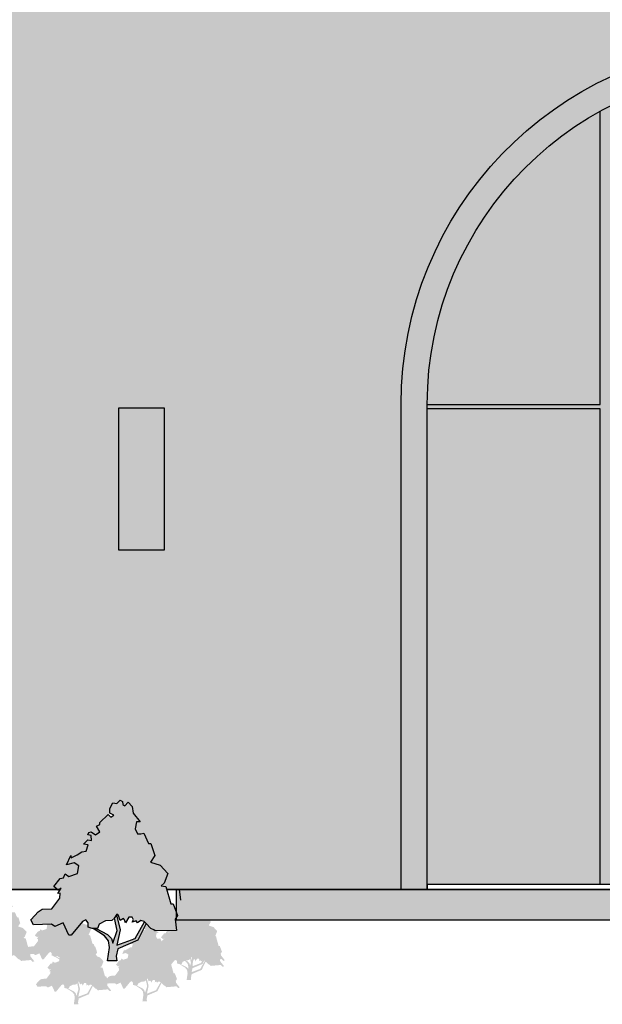
# Model space of a CAD drawing. Units: feet. Extents: x 2368 to 3224, y 836 to 1229.
# Tile 6 of 9: x 2515 to 2603, y 836 to 985. Entities that reach past the tile are written whole.
import ezdxf

# ---------------------------------------------------------------- set-up
doc = ezdxf.new("R2010")
doc.units = ezdxf.units.FT
for name, color, linetype, lineweight in [('A-ELEV', 7, 'Continuous', 25), ('A-ELEV-PATT', 8, 'Continuous', 13), ('L-PLNT', 3, 'Continuous', 13)]:
    doc.layers.add(name, color=color, linetype=linetype, lineweight=lineweight)

msp = doc.modelspace()

# ---------------------------------------------------------------- hatches: boundary and pattern name
at = {"layer": 'A-ELEV-PATT'}
h = msp.add_hatch(color=256, dxfattribs=at)
h.dxf.hatch_style = 1
h.paths.add_polyline_path([(2584.6, 1202.15), (2582.11, 1202.15), (2582.11, 1108.75), (2584.6, 1108.75)])
h.paths.add_polyline_path([(2656.21, 1202.15), (2653.72, 1202.15), (2653.72, 1108.75), (2656.21, 1108.75)])
h.paths.add_polyline_path([(2693.73, 1040.78), (2656.21, 1040.78), (2656.21, 1099.51), (2653.72, 1099.51), (2653.72, 1040.78), (2584.6, 1040.78), (2584.6, 1099.51), (2582.11, 1099.51), (2582.11, 1040.78), (2544.98, 1040.78), (2544.98, 1040.06), (2582.11, 1040.06), (2582.11, 1037.14), (2544.98, 1037.14), (2544.98, 1036.77), (2582.11, 1036.77), (2582.11, 1033.48), (2544.98, 1033.48), (2544.98, 1033.11), (2582.11, 1033.11), (2582.11, 1029.83), (2544.98, 1029.83), (2544.98, 1029.46), (2582.11, 1029.46), (2582.11, 1026.18), (2544.98, 1026.18), (2544.98, 1025.81), (2582.11, 1025.81), (2582.11, 1022.52), (2544.98, 1022.52), (2544.98, 1022.15), (2582.11, 1022.15), (2582.11, 1018.87), (2544.98, 1018.87), (2544.98, 1018.5), (2582.11, 1018.5), (2582.11, 1015.21), (2544.98, 1015.21), (2544.98, 1014.84), (2582.11, 1014.84), (2582.11, 1011.56), (2544.98, 1011.56), (2544.98, 1011.19), (2582.11, 1011.19), (2582.11, 1007.9), (2544.98, 1007.9), (2544.98, 1007.53), (2582.11, 1007.53), (2582.11, 1006.11), (2584.6, 1006.11), (2584.6, 1007.53), (2619.49, 1007.53), (2619.49, 1006.11), (2620.43, 1006.11), (2620.43, 1007.53), (2653.72, 1007.53), (2653.72, 1006.11), (2656.21, 1006.11), (2656.21, 1007.53), (2693.73, 1007.53), (2693.73, 1007.9), (2656.21, 1007.9), (2656.21, 1011.19), (2693.73, 1011.19), (2693.73, 1011.56), (2656.21, 1011.56), (2656.21, 1014.84), (2693.73, 1014.84), (2693.73, 1015.21), (2656.21, 1015.21), (2656.21, 1018.5), (2693.73, 1018.5), (2693.73, 1018.87), (2656.21, 1018.87), (2656.21, 1022.15), (2693.73, 1022.15), (2693.73, 1022.52), (2656.21, 1022.52), (2656.21, 1025.81), (2693.73, 1025.81), (2693.73, 1026.18), (2656.21, 1026.18), (2656.21, 1029.46), (2693.73, 1029.46), (2693.73, 1029.83), (2656.21, 1029.83), (2656.21, 1033.11), (2693.73, 1033.11), (2693.73, 1033.48), (2656.21, 1033.48), (2656.21, 1036.77), (2693.73, 1036.77), (2693.73, 1037.14), (2656.21, 1037.14), (2656.21, 1040.06), (2693.73, 1040.06)])
h.paths.add_polyline_path([(2584.6, 1040.06), (2619.49, 1040.06), (2619.49, 1037.14), (2584.6, 1037.14)], flags=16)
h.paths.add_polyline_path([(2584.6, 1036.77), (2619.49, 1036.77), (2619.49, 1033.48), (2584.6, 1033.48)], flags=16)
h.paths.add_polyline_path([(2584.6, 1033.11), (2619.49, 1033.11), (2619.49, 1029.83), (2584.6, 1029.83)], flags=16)
h.paths.add_polyline_path([(2584.6, 1029.46), (2619.49, 1029.46), (2619.49, 1026.18), (2584.6, 1026.18)], flags=16)
h.paths.add_polyline_path([(2584.6, 1025.81), (2619.49, 1025.81), (2619.49, 1022.52), (2584.6, 1022.52)], flags=16)
h.paths.add_polyline_path([(2584.6, 1022.15), (2619.49, 1022.15), (2619.49, 1018.87), (2584.6, 1018.87)], flags=16)
h.paths.add_polyline_path([(2584.6, 1018.5), (2619.49, 1018.5), (2619.49, 1015.21), (2584.6, 1015.21)], flags=16)
h.paths.add_polyline_path([(2584.6, 1014.84), (2619.49, 1014.84), (2619.49, 1011.56), (2584.6, 1011.56)], flags=16)
h.paths.add_polyline_path([(2584.6, 1011.19), (2619.49, 1011.19), (2619.49, 1007.9), (2584.6, 1007.9)], flags=16)
h.paths.add_polyline_path([(2620.43, 1040.06), (2653.72, 1040.06), (2653.72, 1037.14), (2620.43, 1037.14)], flags=16)
h.paths.add_polyline_path([(2620.43, 1036.77), (2653.72, 1036.77), (2653.72, 1033.48), (2620.43, 1033.48)], flags=16)
h.paths.add_polyline_path([(2620.43, 1033.11), (2653.72, 1033.11), (2653.72, 1029.83), (2620.43, 1029.83)], flags=16)
h.paths.add_polyline_path([(2620.43, 1029.46), (2653.72, 1029.46), (2653.72, 1026.18), (2620.43, 1026.18)], flags=16)
h.paths.add_polyline_path([(2620.43, 1025.81), (2653.72, 1025.81), (2653.72, 1022.52), (2620.43, 1022.52)], flags=16)
h.paths.add_polyline_path([(2620.43, 1022.15), (2653.72, 1022.15), (2653.72, 1018.87), (2620.43, 1018.87)], flags=16)
h.paths.add_polyline_path([(2620.43, 1018.5), (2653.72, 1018.5), (2653.72, 1015.21), (2620.43, 1015.21)], flags=16)
h.paths.add_polyline_path([(2620.43, 1014.84), (2653.72, 1014.84), (2653.72, 1011.56), (2620.43, 1011.56)], flags=16)
h.paths.add_polyline_path([(2620.43, 1011.19), (2653.72, 1011.19), (2653.72, 1007.9), (2620.43, 1007.9)], flags=16)
h.paths.add_polyline_path([(2536.7, 926.19), (2529.87, 926.19), (2529.87, 904.71), (2536.7, 904.71)])
h.paths.add_polyline_path([(2422.21, 920.11), (2416.4, 920.11), (2416.4, 905.78), (2422.21, 905.78)])
h = msp.add_hatch(color=256, dxfattribs=at)
h.dxf.hatch_style = 1
h.paths.add_polyline_path([(2452.58, 1176.09), (2421.63, 1176.09), (2421.63, 1113.35), (2452.58, 1113.35)])
h.paths.add_polyline_path([(2483.52, 1113.35), (2452.58, 1113.35), (2452.58, 1050.6), (2483.52, 1050.6)])
h.paths.add_polyline_path([(2452.58, 1050.6), (2421.63, 1050.6), (2421.63, 987.86), (2452.58, 987.86)])
h.paths.add_polyline_path([(2536.7, 926.19), (2536.7, 904.71), (2529.87, 904.71), (2529.87, 926.19)], flags=16)
h.paths.add_polyline_path([(2719.16, 1202.15), (2694.93, 1202.15), (2694.93, 1108.75), (2694.93, 1002.87), (2696.85, 1002.87), (2696.85, 987.86), (2719.16, 987.86)])
h = msp.add_hatch(color=256, dxfattribs=at)
h.dxf.hatch_style = 1
h.paths.add_polyline_path([(2582.11, 1191.22), (2544.98, 1191.22), (2544.98, 1108.75), (2582.11, 1108.75)])
h.paths.add_polyline_path([(2653.72, 1191.22), (2584.6, 1191.22), (2584.6, 1108.75), (2653.72, 1108.75)])
h.paths.add_polyline_path([(2693.73, 1191.22), (2656.21, 1191.22), (2656.21, 1108.75), (2693.73, 1108.75)])
h.paths.add_polyline_path([(2653.72, 1099.51), (2584.6, 1099.51), (2584.6, 1040.78), (2653.72, 1040.78)])
h.paths.add_polyline_path([(2693.73, 1099.51), (2656.21, 1099.51), (2656.21, 1040.78), (2693.73, 1040.78)])
h.paths.add_polyline_path([(2582.11, 1099.51), (2544.98, 1099.51), (2544.98, 1040.78), (2582.11, 1040.78)])
h.paths.add_polyline_path([(2582.11, 1036.77), (2544.98, 1036.77), (2544.98, 1033.48), (2582.11, 1033.48)])
h.paths.add_polyline_path([(2582.11, 1033.11), (2544.98, 1033.11), (2544.98, 1029.83), (2582.11, 1029.83)])
h.paths.add_polyline_path([(2582.11, 1029.46), (2544.98, 1029.46), (2544.98, 1026.18), (2582.11, 1026.18)])
h.paths.add_polyline_path([(2582.11, 1025.81), (2544.98, 1025.81), (2544.98, 1022.52), (2582.11, 1022.52)])
h.paths.add_polyline_path([(2582.11, 1022.15), (2544.98, 1022.15), (2544.98, 1018.87), (2582.11, 1018.87)])
h.paths.add_polyline_path([(2582.11, 1018.5), (2544.98, 1018.5), (2544.98, 1015.21), (2582.11, 1015.21)])
h.paths.add_polyline_path([(2582.11, 1007.53), (2544.98, 1007.53), (2544.98, 1006.11), (2582.11, 1006.11)])
h.paths.add_polyline_path([(2582.11, 1011.19), (2544.98, 1011.19), (2544.98, 1007.9), (2582.11, 1007.9)])
h.paths.add_polyline_path([(2582.11, 1014.84), (2544.98, 1014.84), (2544.98, 1011.56), (2582.11, 1011.56)])
h.paths.add_polyline_path([(2619.49, 1007.53), (2584.6, 1007.53), (2584.6, 1006.11), (2619.49, 1006.11)])
h.paths.add_polyline_path([(2619.49, 1011.19), (2584.6, 1011.19), (2584.6, 1007.9), (2619.49, 1007.9)])
h.paths.add_polyline_path([(2619.49, 1014.84), (2584.6, 1014.84), (2584.6, 1011.56), (2619.49, 1011.56)])
h.paths.add_polyline_path([(2619.49, 1018.5), (2584.6, 1018.5), (2584.6, 1015.21), (2619.49, 1015.21)])
h.paths.add_polyline_path([(2619.49, 1022.15), (2584.6, 1022.15), (2584.6, 1018.87), (2619.49, 1018.87)])
h.paths.add_polyline_path([(2619.49, 1025.81), (2584.6, 1025.81), (2584.6, 1022.52), (2619.49, 1022.52)])
h.paths.add_polyline_path([(2619.49, 1029.46), (2584.6, 1029.46), (2584.6, 1026.18), (2619.49, 1026.18)])
h.paths.add_polyline_path([(2619.49, 1033.11), (2584.6, 1033.11), (2584.6, 1029.83), (2619.49, 1029.83)])
h.paths.add_polyline_path([(2619.49, 1036.77), (2584.6, 1036.77), (2584.6, 1033.48), (2619.49, 1033.48)])
h.paths.add_polyline_path([(2582.11, 1040.06), (2544.98, 1040.06), (2544.98, 1037.14), (2582.11, 1037.14)])
h.paths.add_polyline_path([(2619.49, 1040.06), (2584.6, 1040.06), (2584.6, 1037.14), (2619.49, 1037.14)])
h.paths.add_polyline_path([(2653.72, 1040.06), (2620.43, 1040.06), (2620.43, 1037.14), (2653.72, 1037.14)])
h.paths.add_polyline_path([(2653.72, 1036.77), (2620.43, 1036.77), (2620.43, 1033.48), (2653.72, 1033.48)])
h.paths.add_polyline_path([(2653.72, 1033.11), (2620.43, 1033.11), (2620.43, 1029.83), (2653.72, 1029.83)])
h.paths.add_polyline_path([(2653.72, 1029.46), (2620.43, 1029.46), (2620.43, 1026.18), (2653.72, 1026.18)])
h.paths.add_polyline_path([(2653.72, 1025.81), (2620.43, 1025.81), (2620.43, 1022.52), (2653.72, 1022.52)])
h.paths.add_polyline_path([(2653.72, 1022.15), (2620.43, 1022.15), (2620.43, 1018.87), (2653.72, 1018.87)])
h.paths.add_polyline_path([(2653.72, 1018.5), (2620.43, 1018.5), (2620.43, 1015.21), (2653.72, 1015.21)])
h.paths.add_polyline_path([(2653.72, 1011.19), (2620.43, 1011.19), (2620.43, 1007.9), (2653.72, 1007.9)])
h.paths.add_polyline_path([(2653.72, 1014.84), (2620.43, 1014.84), (2620.43, 1011.56), (2653.72, 1011.56)])
h.paths.add_polyline_path([(2653.72, 1007.53), (2620.43, 1007.53), (2620.43, 1006.11), (2653.72, 1006.11)])
h.paths.add_polyline_path([(2693.73, 1007.53), (2656.21, 1007.53), (2656.21, 1006.11), (2693.73, 1006.11)])
h.paths.add_polyline_path([(2693.73, 1011.19), (2656.21, 1011.19), (2656.21, 1007.9), (2693.73, 1007.9)])
h.paths.add_polyline_path([(2693.73, 1014.84), (2656.21, 1014.84), (2656.21, 1011.56), (2693.73, 1011.56)])
h.paths.add_polyline_path([(2693.73, 1018.5), (2656.21, 1018.5), (2656.21, 1015.21), (2693.73, 1015.21)])
h.paths.add_polyline_path([(2693.73, 1022.15), (2656.21, 1022.15), (2656.21, 1018.87), (2693.73, 1018.87)])
h.paths.add_polyline_path([(2693.73, 1025.81), (2656.21, 1025.81), (2656.21, 1022.52), (2693.73, 1022.52)])
h.paths.add_polyline_path([(2693.73, 1029.46), (2656.21, 1029.46), (2656.21, 1026.18), (2693.73, 1026.18)])
h.paths.add_polyline_path([(2693.73, 1033.11), (2656.21, 1033.11), (2656.21, 1029.83), (2693.73, 1029.83)])
h.paths.add_polyline_path([(2693.73, 1040.06), (2656.21, 1040.06), (2656.21, 1037.14), (2693.73, 1037.14)])
h.paths.add_polyline_path([(2693.73, 1036.77), (2656.21, 1036.77), (2656.21, 1033.48), (2693.73, 1033.48)])
h.paths.add_polyline_path([(2510.02, 968.65), (2451.35, 968.65), (2451.35, 916.99), (2510.02, 916.99)])
h.paths.add_polyline_path([(2510.02, 916.99), (2470.8, 916.99), (2470.8, 861.76), (2510.02, 861.76)])
h.paths.add_polyline_path([(2650.82, 971.36, 0.250141), (2603.19, 971.36), (2603.19, 926.73), (2650.82, 926.73)])
h.paths.add_polyline_path([(2651.5, 971), (2651.5, 926.73), (2677.6, 926.73, 0.272847)])
h.paths.add_polyline_path([(2677.6, 926.06), (2651.5, 926.06), (2651.5, 854.24), (2677.6, 854.24)])
h.paths.add_polyline_path([(2650.82, 926.06), (2603.19, 926.06), (2603.19, 854.24), (2650.82, 854.24)])
h.paths.add_polyline_path([(2602.51, 971, 0.272847), (2576.42, 926.73), (2602.51, 926.73)])
h.paths.add_polyline_path([(2602.51, 926.06), (2576.42, 926.06), (2576.42, 854.24), (2602.51, 854.24)])
h = msp.add_hatch(color=256, dxfattribs=at)
h.dxf.hatch_style = 1
h.paths.add_polyline_path([(2624.92, 981.22), (2624.92, 981.73, -0.018787), (2629.09, 981.73), (2629.09, 981.22, -0.403049), (2681.53, 926.73), (2681.53, 853.51), (2701.14, 853.51), (2719.16, 853.51), (2719.16, 987.86), (2694.93, 987.86), (2544.98, 987.86), (2510.02, 987.86), (2510.02, 853.51), (2520.58, 853.51), (2520.05, 853.96), (2521, 855.17), (2521.51, 855.27), (2521.73, 855.83), (2522.31, 855.46), (2523.63, 855.92), (2523.84, 857.04), (2523.12, 857.51), (2521.95, 857.23), (2522.6, 858.63), (2522.68, 858.26), (2523.55, 858.73), (2524.28, 859.19), (2524.94, 859.29), (2525.23, 860.22), (2524.5, 860.32), (2525.17, 860.97), (2525.74, 860.88), (2525.67, 861.62), (2525.16, 861.72), (2525.3, 862.09), (2525.67, 862.19), (2526.32, 861.72), (2526.98, 862.19), (2526.47, 863.03), (2526.98, 863.31), (2526.98, 863.59), (2528.51, 865.09), (2528.51, 865.74), (2528.95, 866.58), (2529.53, 866.48), (2530.04, 866.95), (2530.41, 866.77), (2530.48, 866.3), (2530.77, 866.11), (2531.28, 866.67), (2531.86, 866.03), (2532.01, 864.99), (2533.1, 863.68), (2532.52, 863.68), (2532.3, 862.65), (2532.67, 861.9), (2533.18, 861.9), (2533.61, 862), (2534.34, 860.41), (2534.71, 860.41), (2535.29, 858.63), (2534.63, 857.61), (2536.09, 857.14), (2537.26, 855.92), (2536.52, 854.02), (2536.97, 853.96), (2537.09, 853.51), (2572.48, 853.51), (2572.48, 926.73, -0.403049)])
h.paths.add_polyline_path([(2536.7, 926.19), (2536.7, 904.71), (2529.87, 904.71), (2529.87, 926.19)], flags=16)
h = msp.add_hatch(color=256, dxfattribs=at)
h.dxf.hatch_style = 1
h.paths.add_polyline_path([(2624.92, 981.22, 0.403049), (2572.48, 926.73), (2572.48, 853.51), (2576.42, 853.51), (2576.42, 926.73, -0.402184), (2624.92, 977.28)])
h.paths.add_polyline_path([(2629.09, 981.22), (2629.09, 977.28, -0.402184), (2677.6, 926.73), (2677.6, 853.51), (2681.53, 853.51), (2681.53, 926.73, 0.403049)])
h.paths.add_polyline_path([(2629.09, 981.22), (2629.09, 981.73, 0.018787), (2624.92, 981.73), (2624.92, 977.28, -0.020626), (2629.09, 977.28)])
h = msp.add_hatch(color=256, dxfattribs=at)
h.dxf.hatch_style = 1
h.paths.add_polyline_path([(2603.19, 971.36, 0.00378), (2602.51, 971), (2602.51, 926.73), (2576.42, 926.73), (2576.42, 926.06), (2602.51, 926.06), (2602.51, 854.24), (2603.19, 854.24), (2603.19, 926.06), (2650.82, 926.06), (2650.82, 854.24), (2651.5, 854.24), (2651.5, 926.06), (2677.6, 926.06), (2677.6, 926.73), (2651.5, 926.73), (2651.5, 971, 0.00378), (2650.82, 971.36), (2650.82, 926.73), (2603.19, 926.73)])
h = msp.add_hatch(color=256, dxfattribs=at)
h.dxf.hatch_style = 1
h.paths.add_polyline_path([(2536.7, 926.19), (2536.7, 904.71), (2529.87, 904.71), (2529.87, 926.19)], flags=16)
h = msp.add_hatch(color=256, dxfattribs=at)
h.dxf.hatch_style = 1
h.paths.add_polyline_path([(2701.14, 853.51), (2538.51, 853.51), (2538.51, 848.93), (2701.14, 848.93)])
at = {"layer": 'L-PLNT'}
h = msp.add_hatch(color=256, dxfattribs=at)
h.dxf.hatch_style = 1
h.paths.add_polyline_path([(2536.97, 853.96), (2536.24, 854.05), (2536.68, 854.43), (2537.26, 855.92), (2536.09, 857.14), (2534.63, 857.61), (2535.29, 858.63), (2534.71, 860.41), (2534.34, 860.41), (2533.61, 862), (2533.18, 861.9), (2532.67, 861.9), (2532.3, 862.65), (2532.52, 863.68), (2533.1, 863.68), (2532.01, 864.99), (2531.86, 866.03), (2531.28, 866.67), (2530.77, 866.11), (2530.48, 866.3), (2530.41, 866.77), (2530.04, 866.95), (2529.53, 866.48), (2528.95, 866.58), (2528.51, 865.74), (2528.51, 864.99), (2529.09, 864.71), (2528.66, 864.43), (2528.22, 864.8), (2526.98, 863.59), (2526.98, 863.31), (2526.47, 863.03), (2526.98, 862.19), (2526.32, 861.72), (2525.67, 862.19), (2525.3, 862.09), (2525.16, 861.72), (2525.67, 861.62), (2525.74, 860.88), (2525.17, 860.97), (2524.5, 860.32), (2525.23, 860.22), (2524.94, 859.29), (2524.28, 859.19), (2523.55, 858.73), (2522.68, 858.26), (2522.6, 858.63), (2521.95, 857.23), (2523.12, 857.51), (2523.84, 857.04), (2523.63, 855.92), (2522.31, 855.46), (2521.73, 855.83), (2521.51, 855.27), (2521, 855.17), (2520.05, 853.96), (2520.58, 853.51), (2520.88, 853.51), (2521.15, 853.68), (2520.65, 852.87), (2521.01, 852.91), (2520.96, 852.17), (2519.76, 850.59), (2518.3, 850.5), (2517.65, 850.13), (2516.55, 848.91), (2516.99, 848.16), (2519.69, 848.26), (2520.2, 847.88), (2521.44, 848.44), (2522.31, 846.58), (2522.68, 846.58), (2524.35, 848.63), (2524.87, 848.91), (2525.23, 848.44), (2525.23, 847.79), (2525.81, 847.6), (2526.61, 847.6), (2526.91, 848.26), (2527.85, 848.73), (2528.8, 848.82), (2529.22, 849.18), (2529.31, 849.29), (2529.53, 849.75), (2529.82, 849.57), (2530.04, 848.82), (2530.55, 849.1), (2530.7, 848.91), (2530.84, 848.44), (2531.35, 849.29), (2531.86, 849.29), (2532.23, 848.66), (2532.45, 848.73), (2532.67, 848.44), (2533.18, 848.82), (2533.73, 848.61), (2533.72, 848.6), (2533.98, 848.35), (2534.71, 847.6), (2535.15, 847.42), (2535.33, 847.23), (2538.57, 847.32), (2538.35, 849.01), (2538.51, 849.24), (2538.51, 850.13), (2538.06, 851.34), (2537.7, 851.34)])
h = msp.add_hatch(color=256, dxfattribs=at)
h.dxf.hatch_style = 1
h.paths.add_polyline_path([(2515.94, 847.08), (2515.36, 847.68), (2514.64, 847.91), (2514.97, 848.41), (2514.68, 849.29), (2514.5, 849.29), (2514.14, 850.07), (2513.93, 850.03), (2513.67, 850.03), (2513.49, 850.4), (2513.6, 850.9), (2513.89, 850.9), (2513.35, 851.55), (2513.28, 852.06), (2512.99, 852.38), (2512.74, 852.1), (2512.6, 852.19), (2512.56, 852.42), (2512.38, 852.52), (2512.13, 852.29), (2511.84, 852.33), (2511.62, 851.92), (2511.62, 851.55), (2511.91, 851.41), (2511.7, 851.27), (2511.48, 851.46), (2510.87, 850.86), (2510.87, 850.72), (2510.62, 850.58), (2510.69, 850.44), (2510.87, 850.17), (2510.55, 849.94), (2510.22, 850.17), (2510.04, 850.12), (2509.97, 849.94), (2510.22, 849.89), (2510.26, 849.52), (2509.98, 849.57), (2509.65, 849.24), (2510.01, 849.2), (2509.86, 848.74), (2509.54, 848.69), (2509.18, 848.46), (2508.75, 848.23), (2508.71, 848.41), (2508.39, 847.72), (2508.96, 847.86), (2509.32, 847.63), (2509.22, 847.08), (2508.57, 846.85), (2508.28, 847.03), (2508.17, 846.76), (2507.92, 846.71), (2507.71, 846.43), (2507.46, 846.11), (2507.78, 845.83), (2507.99, 845.97), (2507.75, 845.57), (2507.93, 845.59), (2507.9, 845.23), (2507.31, 844.45), (2506.59, 844.41), (2506.27, 844.22), (2505.73, 843.62), (2505.95, 843.25), (2507.28, 843.3), (2507.53, 843.12), (2508.14, 843.39), (2508.57, 842.47), (2508.75, 842.47), (2509.58, 843.48), (2509.83, 843.62), (2510.01, 843.39), (2510.01, 843.07), (2510.29, 842.98), (2510.69, 842.98), (2510.83, 843.3), (2511.3, 843.53), (2511.77, 843.58), (2511.98, 843.76), (2512.02, 843.81), (2512.13, 844.04), (2512.27, 843.94), (2512.38, 843.58), (2512.63, 843.71), (2512.7, 843.62), (2512.78, 843.39), (2513.03, 843.81), (2513.28, 843.81), (2513.39, 843.62), (2513.28, 843.44), (2513.57, 843.53), (2513.67, 843.39), (2513.93, 843.58), (2514.18, 843.48), (2514.68, 842.98), (2514.9, 842.88), (2515.08, 842.7), (2516.59, 842.84), (2516.87, 842.56), (2517.09, 842.65), (2516.51, 843.39), (2516.48, 843.67), (2516.66, 843.94), (2516.33, 844.82), (2516.15, 844.82), (2515.79, 846.11), (2515.43, 846.16), (2515.65, 846.34)])
h = msp.add_hatch(color=256, dxfattribs=at)
h.dxf.hatch_style = 1
h.paths.add_polyline_path([(2525.66, 847.53), (2525.09, 848.13), (2524.37, 848.36), (2524.69, 848.86), (2524.4, 849.74), (2524.22, 849.74), (2523.86, 850.52), (2523.65, 850.48), (2523.4, 850.48), (2523.22, 850.85), (2523.33, 851.35), (2523.61, 851.35), (2523.07, 852), (2523, 852.51), (2522.71, 852.83), (2522.46, 852.55), (2522.32, 852.64), (2522.28, 852.87), (2522.1, 852.97), (2521.85, 852.74), (2521.56, 852.78), (2521.35, 852.37), (2521.35, 852), (2521.64, 851.86), (2521.42, 851.72), (2521.2, 851.91), (2520.59, 851.31), (2520.59, 851.17), (2520.34, 851.03), (2520.41, 850.89), (2520.59, 850.62), (2520.27, 850.39), (2519.95, 850.62), (2519.77, 850.57), (2519.69, 850.39), (2519.95, 850.34), (2519.98, 849.97), (2519.7, 850.02), (2519.37, 849.69), (2519.73, 849.65), (2519.59, 849.19), (2519.26, 849.14), (2518.9, 848.91), (2518.47, 848.68), (2518.44, 848.86), (2518.11, 848.17), (2518.69, 848.31), (2519.05, 848.08), (2518.94, 847.53), (2518.29, 847.3), (2518.01, 847.48), (2517.9, 847.21), (2517.65, 847.16), (2517.43, 846.88), (2517.18, 846.56), (2517.5, 846.28), (2517.72, 846.42), (2517.47, 846.02), (2517.65, 846.04), (2517.63, 845.68), (2517.03, 844.9), (2516.32, 844.86), (2515.99, 844.67), (2515.45, 844.07), (2515.67, 843.7), (2517, 843.75), (2517.25, 843.57), (2517.86, 843.84), (2518.29, 842.92), (2518.47, 842.92), (2519.3, 843.93), (2519.55, 844.07), (2519.73, 843.84), (2519.73, 843.52), (2520.02, 843.43), (2520.41, 843.43), (2520.56, 843.75), (2521.02, 843.98), (2521.49, 844.03), (2521.71, 844.21), (2521.74, 844.26), (2521.85, 844.49), (2522, 844.39), (2522.1, 844.03), (2522.35, 844.16), (2522.43, 844.07), (2522.5, 843.84), (2522.75, 844.26), (2523, 844.26), (2523.11, 844.07), (2523, 843.89), (2523.29, 843.98), (2523.4, 843.84), (2523.65, 844.03), (2523.9, 843.93), (2524.4, 843.43), (2524.62, 843.33), (2524.8, 843.15), (2526.31, 843.29), (2526.6, 843.01), (2526.81, 843.1), (2526.24, 843.84), (2526.2, 844.12), (2526.38, 844.39), (2526.06, 845.27), (2525.88, 845.27), (2525.52, 846.56), (2525.16, 846.61), (2525.37, 846.79)])
h = msp.add_hatch(color=256, dxfattribs=at)
h.dxf.hatch_style = 1
h.paths.add_polyline_path([(2544.71, 847.22), (2544.13, 847.82), (2543.41, 848.05), (2543.73, 848.56), (2543.45, 849.43), (2543.27, 849.43), (2542.91, 850.22), (2542.69, 850.17), (2542.44, 850.17), (2542.26, 850.54), (2542.37, 851.05), (2542.66, 851.05), (2542.12, 851.69), (2542.04, 852.2), (2541.76, 852.52), (2541.51, 852.24), (2541.36, 852.34), (2541.33, 852.57), (2541.15, 852.66), (2540.9, 852.43), (2540.61, 852.47), (2540.39, 852.06), (2540.39, 851.69), (2540.68, 851.55), (2540.46, 851.41), (2540.25, 851.6), (2539.64, 851), (2539.64, 850.86), (2539.39, 850.72), (2539.46, 850.58), (2539.64, 850.31), (2539.31, 850.08), (2538.99, 850.31), (2538.81, 850.26), (2538.74, 850.08), (2538.99, 850.03), (2539.03, 849.66), (2538.74, 849.71), (2538.41, 849.39), (2538.77, 849.34), (2538.63, 848.88), (2538.31, 848.83), (2537.95, 848.6), (2537.52, 848.37), (2537.48, 848.56), (2537.16, 847.87), (2537.73, 848), (2538.09, 847.77), (2537.98, 847.22), (2537.34, 846.99), (2537.05, 847.17), (2536.94, 846.9), (2536.69, 846.85), (2536.47, 846.58), (2536.22, 846.25), (2536.55, 845.98), (2536.76, 846.11), (2536.52, 845.71), (2536.69, 845.73), (2536.67, 845.37), (2536.08, 844.59), (2535.36, 844.55), (2535.04, 844.36), (2534.5, 843.76), (2534.71, 843.4), (2536.04, 843.44), (2536.29, 843.26), (2536.91, 843.53), (2537.34, 842.61), (2537.52, 842.61), (2538.34, 843.63), (2538.59, 843.76), (2538.77, 843.53), (2538.77, 843.21), (2539.06, 843.12), (2539.46, 843.12), (2539.6, 843.44), (2540.07, 843.67), (2540.54, 843.72), (2540.75, 843.9), (2540.79, 843.95), (2540.9, 844.18), (2541.04, 844.09), (2541.15, 843.72), (2541.4, 843.86), (2541.47, 843.76), (2541.54, 843.53), (2541.79, 843.95), (2542.05, 843.95), (2542.15, 843.76), (2542.05, 843.58), (2542.33, 843.67), (2542.44, 843.53), (2542.69, 843.72), (2542.94, 843.63), (2543.45, 843.12), (2543.66, 843.03), (2543.84, 842.84), (2545.35, 842.98), (2545.64, 842.7), (2545.86, 842.8), (2545.28, 843.53), (2545.24, 843.81), (2545.42, 844.09), (2545.1, 844.96), (2544.92, 844.96), (2544.56, 846.25), (2544.2, 846.3), (2544.42, 846.48)])
h = msp.add_hatch(color=256, dxfattribs=at)
h.dxf.hatch_style = 1
h.paths.add_polyline_path([(2544.58, 846.33), (2544.01, 846.93), (2543.29, 847.16), (2543.61, 847.67), (2543.33, 848.54), (2543.15, 848.54), (2542.79, 849.32), (2542.57, 849.28), (2542.32, 849.28), (2542.14, 849.65), (2542.25, 850.15), (2542.54, 850.15), (2542, 850.8), (2541.92, 851.31), (2541.64, 851.63), (2541.39, 851.35), (2541.24, 851.44), (2541.21, 851.67), (2541.03, 851.77), (2540.77, 851.54), (2540.49, 851.58), (2540.27, 851.17), (2540.27, 850.8), (2540.56, 850.66), (2540.34, 850.52), (2540.13, 850.71), (2539.52, 850.11), (2539.52, 849.97), (2539.26, 849.83), (2539.34, 849.69), (2539.52, 849.42), (2539.19, 849.19), (2538.87, 849.42), (2538.69, 849.37), (2538.62, 849.19), (2538.87, 849.14), (2538.91, 848.77), (2538.62, 848.82), (2538.29, 848.49), (2538.65, 848.45), (2538.51, 847.99), (2538.19, 847.94), (2537.83, 847.71), (2537.4, 847.48), (2537.36, 847.67), (2537.04, 846.97), (2537.61, 847.11), (2537.97, 846.88), (2537.86, 846.33), (2537.22, 846.1), (2536.93, 846.28), (2536.82, 846.01), (2536.57, 845.96), (2536.35, 845.68), (2536.1, 845.36), (2536.43, 845.08), (2536.64, 845.22), (2536.4, 844.82), (2536.57, 844.84), (2536.55, 844.48), (2535.96, 843.7), (2535.24, 843.66), (2534.92, 843.47), (2534.38, 842.87), (2534.59, 842.5), (2535.92, 842.55), (2536.17, 842.37), (2536.78, 842.64), (2537.22, 841.72), (2537.4, 841.72), (2538.22, 842.73), (2538.47, 842.87), (2538.65, 842.64), (2538.65, 842.32), (2538.94, 842.23), (2539.34, 842.23), (2539.48, 842.55), (2539.95, 842.78), (2540.42, 842.83), (2540.63, 843.01), (2540.67, 843.06), (2540.77, 843.29), (2540.92, 843.2), (2541.03, 842.83), (2541.28, 842.97), (2541.35, 842.87), (2541.42, 842.64), (2541.67, 843.06), (2541.92, 843.06), (2542.03, 842.87), (2541.92, 842.69), (2542.21, 842.78), (2542.32, 842.64), (2542.57, 842.83), (2542.82, 842.73), (2543.33, 842.23), (2543.54, 842.14), (2543.72, 841.95), (2545.23, 842.09), (2545.52, 841.81), (2545.74, 841.91), (2545.16, 842.64), (2545.12, 842.92), (2545.3, 843.2), (2544.98, 844.07), (2544.8, 844.07), (2544.44, 845.36), (2544.08, 845.41), (2544.3, 845.59)])
h = msp.add_hatch(color=256, dxfattribs=at)
h.dxf.hatch_style = 1
h.paths.add_polyline_path([(2532.74, 845.83), (2533.98, 848.35), (2533.72, 848.6), (2532.3, 846.11), (2529.53, 845.08), (2530.04, 847.42), (2529.49, 849.67), (2529.31, 849.29), (2529.22, 849.17), (2529.6, 847.32), (2528.95, 845.36), (2528.73, 846.11), (2528.15, 846.67), (2526.41, 847.6), (2525.96, 847.6), (2527.71, 846.48), (2528.29, 845.73), (2528.44, 844.71), (2528.15, 842.74), (2529.53, 842.74), (2529.46, 843.4), (2529.68, 844.52)])
h = msp.add_hatch(color=256, dxfattribs=at)
h.dxf.hatch_style = 1
h.paths.add_polyline_path([(2527.55, 842.65), (2526.97, 843.25), (2526.25, 843.48), (2526.58, 843.98), (2526.29, 844.86), (2526.11, 844.86), (2525.75, 845.64), (2525.54, 845.6), (2525.28, 845.6), (2525.1, 845.97), (2525.21, 846.47), (2525.5, 846.47), (2524.96, 847.12), (2524.89, 847.63), (2524.6, 847.95), (2524.35, 847.67), (2524.21, 847.76), (2524.17, 847.99), (2523.99, 848.09), (2523.74, 847.86), (2523.45, 847.9), (2523.23, 847.49), (2523.23, 847.12), (2523.52, 846.98), (2523.31, 846.84), (2523.09, 847.03), (2522.48, 846.43), (2522.48, 846.29), (2522.23, 846.15), (2522.3, 846.01), (2522.48, 845.74), (2522.16, 845.51), (2521.83, 845.74), (2521.65, 845.69), (2521.58, 845.51), (2521.83, 845.46), (2521.87, 845.09), (2521.59, 845.14), (2521.26, 844.81), (2521.62, 844.77), (2521.47, 844.31), (2521.15, 844.26), (2520.79, 844.03), (2520.36, 843.8), (2520.32, 843.98), (2520, 843.29), (2520.57, 843.43), (2520.93, 843.2), (2520.83, 842.65), (2520.18, 842.42), (2519.89, 842.6), (2519.78, 842.33), (2519.53, 842.28), (2519.32, 842), (2519.07, 841.68), (2519.39, 841.4), (2519.6, 841.54), (2519.36, 841.14), (2519.54, 841.16), (2519.51, 840.8), (2518.92, 840.02), (2518.2, 839.98), (2517.88, 839.79), (2517.34, 839.19), (2517.56, 838.82), (2518.89, 838.87), (2519.14, 838.69), (2519.75, 838.96), (2520.18, 838.04), (2520.36, 838.04), (2521.19, 839.05), (2521.44, 839.19), (2521.62, 838.96), (2521.62, 838.64), (2521.9, 838.55), (2522.3, 838.55), (2522.44, 838.87), (2522.91, 839.1), (2523.38, 839.15), (2523.59, 839.33), (2523.63, 839.38), (2523.74, 839.61), (2523.88, 839.51), (2523.99, 839.15), (2524.24, 839.28), (2524.31, 839.19), (2524.39, 838.96), (2524.64, 839.38), (2524.89, 839.38), (2525, 839.19), (2524.89, 839.01), (2525.18, 839.1), (2525.28, 838.96), (2525.54, 839.15), (2525.79, 839.05), (2526.29, 838.55), (2526.51, 838.46), (2526.69, 838.27), (2528.2, 838.41), (2528.48, 838.13), (2528.7, 838.22), (2528.12, 838.96), (2528.09, 839.24), (2528.27, 839.51), (2527.94, 840.39), (2527.76, 840.39), (2527.4, 841.68), (2527.04, 841.73), (2527.26, 841.91)])
h = msp.add_hatch(color=256, dxfattribs=at)
h.dxf.hatch_style = 1
h.paths.add_polyline_path([(2537.91, 843.11), (2537.33, 843.71), (2536.61, 843.94), (2536.94, 844.44), (2536.65, 845.32), (2536.47, 845.32), (2536.11, 846.1), (2535.9, 846.06), (2535.64, 846.06), (2535.46, 846.43), (2535.57, 846.93), (2535.86, 846.93), (2535.32, 847.58), (2535.25, 848.09), (2534.96, 848.41), (2534.71, 848.13), (2534.57, 848.22), (2534.53, 848.45), (2534.35, 848.55), (2534.1, 848.32), (2533.81, 848.36), (2533.59, 847.95), (2533.59, 847.58), (2533.88, 847.44), (2533.67, 847.3), (2533.45, 847.49), (2532.84, 846.89), (2532.84, 846.75), (2532.59, 846.61), (2532.66, 846.47), (2532.84, 846.2), (2532.52, 845.97), (2532.19, 846.2), (2532.01, 846.15), (2531.94, 845.97), (2532.19, 845.92), (2532.23, 845.55), (2531.95, 845.6), (2531.62, 845.27), (2531.98, 845.23), (2531.83, 844.77), (2531.51, 844.72), (2531.15, 844.49), (2530.72, 844.26), (2530.68, 844.44), (2530.36, 843.75), (2530.93, 843.89), (2531.29, 843.66), (2531.19, 843.11), (2530.54, 842.88), (2530.25, 843.06), (2530.14, 842.79), (2529.89, 842.74), (2529.68, 842.46), (2529.43, 842.14), (2529.75, 841.86), (2529.96, 842), (2529.72, 841.6), (2529.9, 841.62), (2529.87, 841.26), (2529.28, 840.48), (2528.56, 840.44), (2528.24, 840.25), (2527.7, 839.65), (2527.92, 839.28), (2529.25, 839.33), (2529.5, 839.15), (2530.11, 839.42), (2530.54, 838.5), (2530.72, 838.5), (2531.55, 839.51), (2531.8, 839.65), (2531.98, 839.42), (2531.98, 839.1), (2532.26, 839.01), (2532.66, 839.01), (2532.8, 839.33), (2533.27, 839.56), (2533.74, 839.61), (2533.95, 839.79), (2533.99, 839.84), (2534.1, 840.07), (2534.24, 839.97), (2534.35, 839.61), (2534.6, 839.74), (2534.67, 839.65), (2534.75, 839.42), (2535, 839.84), (2535.25, 839.84), (2535.36, 839.65), (2535.25, 839.47), (2535.54, 839.56), (2535.64, 839.42), (2535.9, 839.61), (2536.15, 839.51), (2536.65, 839.01), (2536.87, 838.92), (2537.05, 838.73), (2538.56, 838.87), (2538.84, 838.59), (2539.06, 838.68), (2538.48, 839.42), (2538.45, 839.7), (2538.63, 839.97), (2538.3, 840.85), (2538.12, 840.85), (2537.76, 842.14), (2537.41, 842.19), (2537.62, 842.37)])
h = msp.add_hatch(color=256, dxfattribs=at)
h.dxf.hatch_style = 1
h.paths.add_polyline_path([(2521.92, 841.91), (2523.43, 842.55), (2524.04, 843.79), (2523.92, 843.92), (2523.9, 843.89), (2523.22, 842.69), (2521.85, 842.18), (2522.1, 843.33), (2521.85, 844.39), (2521.84, 844.46), (2521.74, 844.26), (2521.71, 844.21), (2521.68, 844.19), (2521.71, 844.16), (2521.89, 843.29), (2521.56, 842.32), (2521.46, 842.69), (2521.17, 842.97), (2520.34, 843.38), (2520.27, 843.43), (2520.09, 843.43), (2520.95, 842.87), (2521.24, 842.51), (2521.31, 842), (2521.17, 841.03), (2521.85, 841.03), (2521.82, 841.35)])
h = msp.add_hatch(color=256, dxfattribs=at)
h.dxf.hatch_style = 1
h.paths.add_polyline_path([(2540.85, 840.71), (2542.36, 841.35), (2542.97, 842.59), (2542.84, 842.72), (2542.82, 842.69), (2542.14, 841.49), (2540.77, 840.98), (2541.03, 842.14), (2540.77, 843.2), (2540.76, 843.26), (2540.67, 843.06), (2540.63, 843.01), (2540.61, 842.99), (2540.63, 842.97), (2540.81, 842.09), (2540.49, 841.12), (2540.38, 841.49), (2540.09, 841.77), (2539.26, 842.18), (2539.19, 842.23), (2539.01, 842.23), (2539.88, 841.67), (2540.16, 841.31), (2540.24, 840.8), (2540.09, 839.83), (2540.77, 839.83), (2540.74, 840.15)])
h = msp.add_hatch(color=256, dxfattribs=at)
h.dxf.hatch_style = 1
h.paths.add_polyline_path([(2540.97, 841.6), (2542.48, 842.24), (2543.09, 843.48), (2542.96, 843.61), (2542.94, 843.58), (2542.26, 842.38), (2540.9, 841.87), (2541.15, 843.03), (2540.9, 844.09), (2540.88, 844.15), (2540.79, 843.95), (2540.75, 843.9), (2540.73, 843.88), (2540.75, 843.86), (2540.93, 842.98), (2540.61, 842.01), (2540.5, 842.38), (2540.21, 842.66), (2539.39, 843.07), (2539.31, 843.12), (2539.13, 843.12), (2540, 842.57), (2540.28, 842.2), (2540.36, 841.69), (2540.21, 840.72), (2540.9, 840.72), (2540.86, 841.05)])
h = msp.add_hatch(color=256, dxfattribs=at)
h.dxf.hatch_style = 1
h.paths.add_polyline_path([(2534.17, 837.49), (2535.68, 838.13), (2536.29, 839.37), (2536.16, 839.5), (2536.15, 839.47), (2535.46, 838.27), (2534.1, 837.76), (2534.35, 838.92), (2534.1, 839.97), (2534.08, 840.04), (2533.99, 839.84), (2533.95, 839.79), (2533.93, 839.77), (2533.95, 839.74), (2534.13, 838.87), (2533.81, 837.9), (2533.7, 838.27), (2533.42, 838.55), (2532.59, 838.96), (2532.52, 839.01), (2532.34, 839.01), (2533.2, 838.45), (2533.49, 838.09), (2533.56, 837.58), (2533.42, 836.61), (2534.1, 836.61), (2534.06, 836.93)])
h = msp.add_hatch(color=256, dxfattribs=at)
h.dxf.hatch_style = 1
h.paths.add_polyline_path([(2523.81, 837.03), (2525.32, 837.67), (2525.93, 838.91), (2525.8, 839.04), (2525.79, 839.01), (2525.1, 837.81), (2523.74, 837.3), (2523.99, 838.46), (2523.74, 839.51), (2523.72, 839.58), (2523.63, 839.38), (2523.59, 839.33), (2523.57, 839.31), (2523.59, 839.28), (2523.77, 838.41), (2523.45, 837.44), (2523.34, 837.81), (2523.06, 838.09), (2522.23, 838.5), (2522.16, 838.55), (2521.98, 838.55), (2522.84, 837.99), (2523.13, 837.63), (2523.2, 837.12), (2523.06, 836.15), (2523.74, 836.15), (2523.7, 836.47)])

# ---------------------------------------------------------------- linework, layer by layer
at = {"layer": 'A-ELEV'}
for p, q in [((2394.91, 853.51), (2521.04, 853.51)), ((2394.91, 853.51), (2521.04, 853.51)), ((2537.09, 853.51), (2719.16, 853.51)), ((2537.09, 853.51), (2719.16, 853.51)), ((2538.97, 853.54), (2539.19, 851.85))]:
    msp.add_line(p, q, dxfattribs=at)
for points in [[(2521.04, 853.51), (2510.02, 853.51), (2510.02, 987.86), (2719.16, 987.86), (2719.16, 853.51), (2537.09, 853.51)], [(2521.04, 853.51), (2510.02, 853.51), (2510.02, 987.86), (2719.16, 987.86), (2719.16, 853.51), (2537.09, 853.51)], [(2602.51, 926.73), (2602.51, 971)], [(2602.51, 926.73), (2602.51, 971)], [(2602.51, 926.06), (2576.42, 926.06), (2576.42, 926.73), (2602.51, 926.73)], [(2602.51, 926.06), (2576.42, 926.06), (2576.42, 926.73), (2602.51, 926.73)], [(2602.51, 854.24), (2602.51, 926.06)], [(2602.51, 854.24), (2602.51, 926.06)]]:
    msp.add_lwpolyline(points, dxfattribs=at)
for points in [[(2572.48, 853.51), (2572.48, 926.73, -0.403049), (2624.92, 981.22, -0.403049)], [(2572.48, 853.51), (2572.48, 926.73, -0.403049), (2624.92, 981.22, -0.403049)], [(2576.42, 853.51), (2576.42, 926.73, -1), (2677.6, 926.73), (2677.6, 853.51)], [(2576.42, 853.51), (2576.42, 926.73, -1), (2677.6, 926.73), (2677.6, 853.51)]]:
    msp.add_lwpolyline(points, format="xyb", dxfattribs=at)
for points in [[(2529.87, 926.19), (2536.7, 926.19), (2536.7, 904.71), (2529.87, 904.71)], [(2529.87, 926.19), (2536.7, 926.19), (2536.7, 904.71), (2529.87, 904.71)], [(2538.57, 847.32), (2535.33, 847.23), (2535.15, 847.42), (2534.71, 847.6), (2533.98, 848.35), (2533.69, 848.63), (2533.18, 848.82), (2532.67, 848.44), (2532.45, 848.73), (2531.86, 848.54), (2532.08, 848.91), (2531.86, 849.29), (2531.35, 849.29), (2530.84, 848.44), (2530.7, 848.91), (2530.55, 849.1), (2530.04, 848.82), (2529.82, 849.57), (2529.53, 849.75), (2529.31, 849.29), (2529.24, 849.19), (2528.8, 848.82), (2527.85, 848.73), (2526.91, 848.26), (2526.61, 847.6), (2525.81, 847.6), (2525.23, 847.79), (2525.23, 848.44), (2524.87, 848.91), (2524.35, 848.63), (2522.68, 846.58), (2522.31, 846.58), (2521.44, 848.44), (2520.2, 847.88), (2519.69, 848.26), (2516.99, 848.16), (2516.55, 848.91), (2516.61, 848.98), (2517.65, 850.13), (2518.3, 850.5), (2519.76, 850.59), (2520.96, 852.17), (2521.01, 852.91), (2520.65, 852.87), (2521.15, 853.68), (2520.71, 853.4), (2520.05, 853.96), (2521, 855.17), (2521.51, 855.27), (2521.73, 855.83), (2522.31, 855.46), (2523.63, 855.92), (2523.84, 857.04), (2523.12, 857.51), (2521.95, 857.23), (2522.6, 858.63), (2522.68, 858.26), (2523.55, 858.73), (2524.28, 859.19), (2524.94, 859.29), (2525.23, 860.22), (2524.5, 860.32), (2525.17, 860.97), (2525.74, 860.88), (2525.67, 861.62), (2525.16, 861.72), (2525.3, 862.09), (2525.67, 862.19), (2526.32, 861.72), (2526.98, 862.19), (2526.47, 863.03), (2526.98, 863.31), (2526.98, 863.59), (2528.22, 864.8), (2528.66, 864.43), (2529.09, 864.71), (2528.51, 864.99), (2528.51, 865.74), (2528.95, 866.58), (2529.53, 866.48), (2530.04, 866.95), (2530.41, 866.77), (2530.48, 866.3), (2530.77, 866.11), (2531.28, 866.67), (2531.86, 866.03), (2532.01, 864.99), (2533.1, 863.68), (2532.52, 863.68), (2532.3, 862.65), (2532.67, 861.9), (2533.18, 861.9), (2533.61, 862), (2534.34, 860.41), (2534.71, 860.41), (2535.29, 858.63), (2534.63, 857.61), (2536.09, 857.14), (2537.26, 855.92), (2536.68, 854.43), (2536.24, 854.05), (2536.97, 853.96), (2537.7, 851.34), (2538.06, 851.34), (2538.72, 849.57), (2538.35, 849.01)], [(2538.57, 847.32), (2535.33, 847.23), (2535.15, 847.42), (2534.71, 847.6), (2533.98, 848.35), (2533.69, 848.63), (2533.18, 848.82), (2532.67, 848.44), (2532.45, 848.73), (2531.86, 848.54), (2532.08, 848.91), (2531.86, 849.29), (2531.35, 849.29), (2530.84, 848.44), (2530.7, 848.91), (2530.55, 849.1), (2530.04, 848.82), (2529.82, 849.57), (2529.53, 849.75), (2529.31, 849.29), (2529.24, 849.19), (2528.8, 848.82), (2527.85, 848.73), (2526.91, 848.26), (2526.61, 847.6), (2525.81, 847.6), (2525.23, 847.79), (2525.23, 848.44), (2524.87, 848.91), (2524.35, 848.63), (2522.68, 846.58), (2522.31, 846.58), (2521.44, 848.44), (2520.2, 847.88), (2519.69, 848.26), (2516.99, 848.16), (2516.55, 848.91), (2516.61, 848.98), (2517.65, 850.13), (2518.3, 850.5), (2519.76, 850.59), (2520.96, 852.17), (2521.01, 852.91), (2520.65, 852.87), (2521.15, 853.68), (2520.71, 853.4), (2520.05, 853.96), (2521, 855.17), (2521.51, 855.27), (2521.73, 855.83), (2522.31, 855.46), (2523.63, 855.92), (2523.84, 857.04), (2523.12, 857.51), (2521.95, 857.23), (2522.6, 858.63), (2522.68, 858.26), (2523.55, 858.73), (2524.28, 859.19), (2524.94, 859.29), (2525.23, 860.22), (2524.5, 860.32), (2525.17, 860.97), (2525.74, 860.88), (2525.67, 861.62), (2525.16, 861.72), (2525.3, 862.09), (2525.67, 862.19), (2526.32, 861.72), (2526.98, 862.19), (2526.47, 863.03), (2526.98, 863.31), (2526.98, 863.59), (2528.22, 864.8), (2528.66, 864.43), (2529.09, 864.71), (2528.51, 864.99), (2528.51, 865.74), (2528.95, 866.58), (2529.53, 866.48), (2530.04, 866.95), (2530.41, 866.77), (2530.48, 866.3), (2530.77, 866.11), (2531.28, 866.67), (2531.86, 866.03), (2532.01, 864.99), (2533.1, 863.68), (2532.52, 863.68), (2532.3, 862.65), (2532.67, 861.9), (2533.18, 861.9), (2533.61, 862), (2534.34, 860.41), (2534.71, 860.41), (2535.29, 858.63), (2534.63, 857.61), (2536.09, 857.14), (2537.26, 855.92), (2536.68, 854.43), (2536.24, 854.05), (2536.97, 853.96), (2537.7, 851.34), (2538.06, 851.34), (2538.72, 849.57), (2538.35, 849.01)], [(2701.14, 853.51), (2538.51, 853.51), (2538.51, 848.93), (2701.14, 848.93)], [(2701.14, 853.51), (2538.51, 853.51), (2538.51, 848.93), (2701.14, 848.93)], [(2576.42, 853.51), (2677.6, 853.51), (2677.6, 854.24), (2576.42, 854.24)], [(2576.42, 853.51), (2677.6, 853.51), (2677.6, 854.24), (2576.42, 854.24)], [(2529.22, 849.18), (2529.31, 849.29), (2529.49, 849.67), (2530.04, 847.42), (2529.53, 845.08), (2532.3, 846.11), (2533.72, 848.6), (2533.98, 848.35), (2532.74, 845.83), (2529.68, 844.52), (2529.46, 843.4), (2529.53, 842.74), (2528.15, 842.74), (2528.44, 844.71), (2528.29, 845.73), (2527.71, 846.48), (2525.96, 847.6), (2526.41, 847.6), (2528.15, 846.67), (2528.73, 846.11), (2528.95, 845.36), (2529.6, 847.32)]]:
    msp.add_lwpolyline(points, close=True, dxfattribs=at)

doc.saveas('drawing.dxf')
